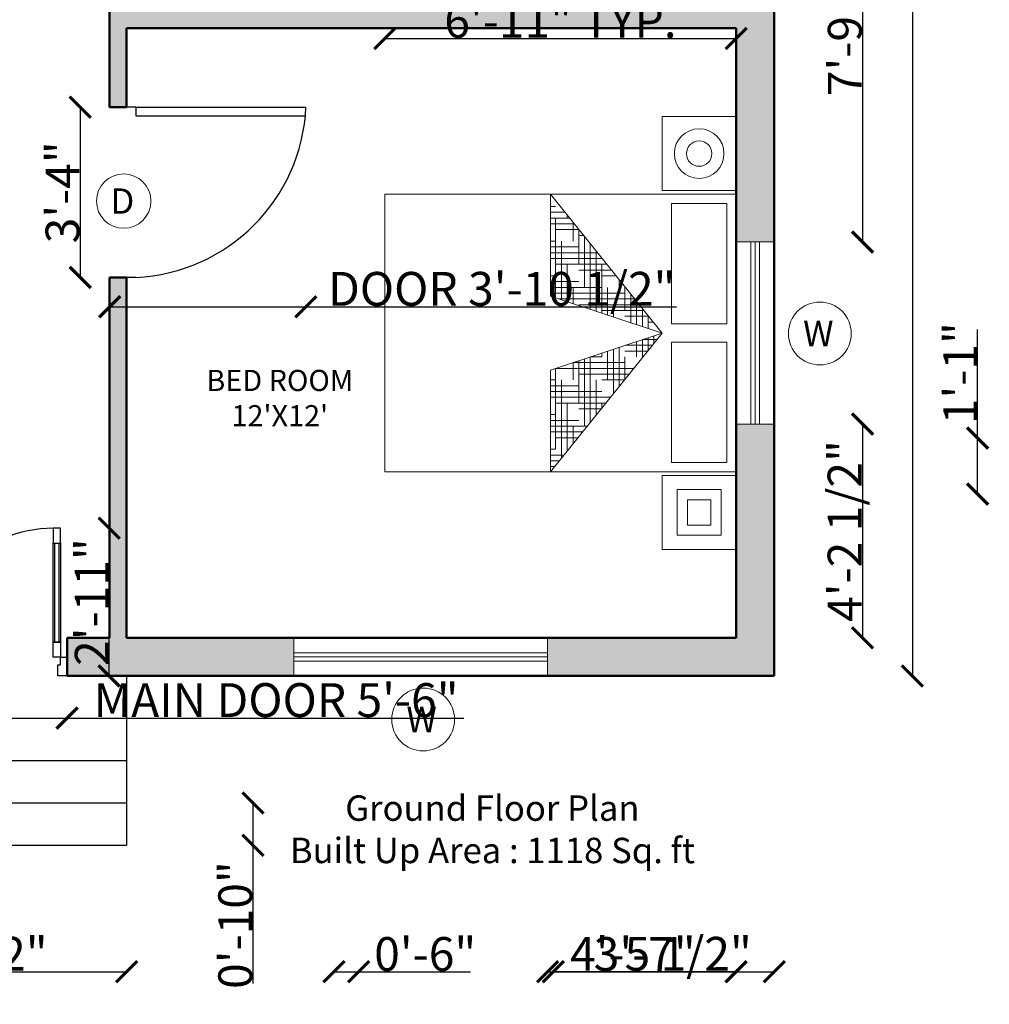
# Model space of a CAD drawing. Units: inches. Extents: x 2169 to 2662, y 1518 to 2151.
# Tile 3 of 6: x 2398 to 2627, y 1518 to 1751. Entities that reach past the tile are written whole.
import ezdxf

# ---------------------------------------------------------------- set-up
doc = ezdxf.new("R2010")
doc.units = ezdxf.units.IN
for name, color, linetype, lineweight in [('A-ANNO-DIMS', 2, 'Continuous', 18), ('A-ANNO-SYMB', 7, 'Continuous', 18), ('A-ANNO-TEXT', 7, 'Continuous', 18), ('A-AREA-IDEN', 7, 'Continuous', 18), ('A-FURN', 8, 'Continuous', 18), ('A-WALL-PATT', 30, 'Continuous', 13), ('Doors', 240, 'Continuous', 30), ('Main Door', 150, 'Continuous', 30), ('Steps', 50, 'Continuous', 25), ('Walls', 7, 'Continuous', 50), ('Windows', 160, 'Continuous', 18)]:
    doc.layers.add(name, color=color, linetype=linetype, lineweight=lineweight)
doc.layers.add('A-Glaz', color=92, linetype='Continuous')
doc.styles.get("Standard").update_dxf_attribs({"font": 'arial.ttf'})
doc.dimstyles.get("Standard").update_dxf_attribs({"dimtxt": 8, "dimasz": 5, "dimexe": 0.18, "dimexo": 0.0625, "dimgap": 0.09, "dimtad": 1, "dimdec": 1, "dimzin": 0, "dimdsep": 46, "dimlunit": 4, "dimtxsty": 'Standard', "dimblk": 'ARCHTICK', "dimcen": 0.09, "dimse1": 1, "dimse2": 1, "dimadec": 0, "dimazin": 0, "dimtfac": 1, "dimtdec": 1, "dimtofl": 0, "dimtmove": 0, "dimatfit": 3, "dimfxl": 1, "dimtolj": 1, "dimtzin": 0, "dimarcsym": 0})

# ---------------------------------------------------------------- blocks, each defined once
blk = doc.blocks.new('_ArchTick')
at = {"color": 0, "linetype": 'ByBlock', "const_width": 0.15}
blk.add_lwpolyline([(-0.5, -0.5), (0.5, 0.5)], dxfattribs=at)
blk = doc.blocks.new('*D3')
at = {"layer": 'A-ANNO-DIMS', "color": 0, "lineweight": -2, "transparency": 16777216}
blk.add_line((2608.61, 2111.6), (2608.61, 1595.6), dxfattribs=at)
at = {"layer": 'Defpoints', "color": 0, "transparency": 16777216}
for p in [(2575.74, 2111.6), (2575.98, 1595.6), (2608.61, 1595.6)]:
    blk.add_point(p, dxfattribs=at)
at = {"layer": 'A-ANNO-DIMS', "color": 0, "lineweight": -2, "transparency": 16777216, "xscale": 5, "yscale": 5, "zscale": 5}
for p, rotation in [((2608.61, 2111.6), 90), ((2608.61, 1595.6), 270)]:
    blk.add_blockref('_ArchTick', p, dxfattribs=dict(at, rotation=rotation))
at = {"layer": 'A-ANNO-DIMS', "color": 0, "transparency": 16777216, "insert": (2604.43, 1853.6), "char_height": 8, "attachment_point": 5, "rotation": 90}
blk.add_mtext("\\A1;43'", dxfattribs=at)
blk = doc.blocks.new('A$C13CE0A17')
at = {"layer": 'A-Glaz'}
for p, q in [((0.01, 0.61), (0.01, 0.08)), ((0.03, 0.08), (0.03, 0.61))]:
    blk.add_line(p, q, dxfattribs=at)
blk.add_lwpolyline([(1.4, 0.08), (1.4, 0.61), (1.42, 0.61), (1.42, 0.08)], close=True, dxfattribs=at)
at = {"layer": 'Main Door'}
for p, q in [((0, 0.61), (0, 0.69)), ((0, 0.69), (0.04, 0.69)), ((0.04, 0.69), (0.04, 0.61)), ((0, 0.61), (0, 0.08)), ((0.04, 0.61), (0, 0.61)), ((0.04, 0.61), (0, 0.61)), ((0.03, 0.61), (0.01, 0.61)), ((0.04, 0.08), (0.04, 0.61)), ((0, 0.08), (0, 0)), ((0.04, 0.08), (0, 0.08)), ((0, 0.08), (0.04, 0.08)), ((0.01, 0.08), (0.03, 0.08)), ((0.04, 0), (0.04, 0.08)), ((-0.035, 0), (-0.035, -0.1)), ((0, 0), (-0.035, 0)), ((0, 0), (0.04, 0)), ((0, -0.04), (0, 0)), ((0.015, -0.04), (0, -0.04)), ((0.015, -0.05), (0.015, -0.04)), ((0.015, -0.1), (0.015, -0.05)), ((-0.035, -0.1), (0.015, -0.1))]:
    blk.add_line(p, q, dxfattribs=at)
for points in [[(1.39, 0.69), (1.39, 0.61), (1.43, 0.61), (1.43, 0.69)], [(1.39, 0.08), (1.39, 0.61), (1.43, 0.61), (1.43, 0.08)], [(1.39, 0), (1.39, 0.08), (1.43, 0.08), (1.43, 0)], [(1.43, 0), (1.465, 0), (1.465, -0.1), (1.415, -0.1), (1.415, -0.05), (1.415, -0.04), (1.43, -0.04)]]:
    blk.add_lwpolyline(points, close=True, dxfattribs=at)
blk.add_arc((1.3872, 0.017), 0.673, 89.7657, 181.4438, dxfattribs=at)
blk.add_ellipse((0.0389, 0.0511), major_axis=(0.6669, -0.1217), ratio=0.940794, start_param=0.11153, end_param=1.73917, dxfattribs=at)
blk = doc.blocks.new('*X16')
at = {"color": 0}
for p, q in [((20.25, 14.8125), (20.2772, 14.8125)), ((20.1739, 14.75), (20.2772, 14.75)), ((20.1875, 14.75), (20.1875, 14.7669)), ((20.199, 14.7812), (20.2772, 14.7812)), ((20.25, 14.3194), (20.25, 14.75)), ((20.1487, 14.7188), (20.2772, 14.7188)), ((20.1562, 14.625), (20.1562, 14.7281)), ((20.0938, 14.375), (20.0938, 14.6504)), ((20.0984, 14.6562), (20.125, 14.6562)), ((20.1236, 14.6875), (20.25, 14.6875)), ((20.125, 14.5), (20.125, 14.6893)), ((20.0625, 14.2573), (20.0625, 14.6116)), ((20.125, 14.5938), (20.2772, 14.5938)), ((20.2188, 14.3091), (20.2188, 14.625)), ((20.25, 14.625), (20.2772, 14.625)), ((20.023, 14.5625), (20.2772, 14.5625)), ((20.0312, 14.2469), (20.0312, 14.5727)), ((19.9727, 14.5), (20.25, 14.5)), ((19.9979, 14.5312), (20.2772, 14.5312)), ((20, 14.2366), (20, 14.5)), ((20.1875, 14.2987), (20.1875, 14.5)), ((19.9225, 14.4375), (20, 14.4375)), ((19.9476, 14.4688), (20.125, 14.4688)), ((20.25, 14.4375), (20.2772, 14.4375)), ((19.875, 14.25), (19.875, 14.3785)), ((19.9062, 14.375), (19.9062, 14.4174)), ((19.9688, 14.2262), (19.9688, 14.375)), ((20, 14.375), (20.2772, 14.375)), ((20.125, 14.4062), (20.2772, 14.4062)), ((20.1562, 14.2884), (20.1562, 14.375)), ((19.8438, 14.1848), (19.8438, 14.3397)), ((19.875, 14.3438), (20.2772, 14.3438)), ((19.7967, 14.2812), (20.125, 14.2812)), ((19.8125, 14.1744), (19.8125, 14.3008)), ((19.8219, 14.3125), (20.2291, 14.3125)), ((19.7465, 14.2188), (19.875, 14.2188)), ((19.75, 14.1537), (19.75, 14.2231)), ((19.7716, 14.25), (20, 14.25)), ((19.7812, 14.1641), (19.7812, 14.262)), ((19.9375, 14.2159), (19.9375, 14.25)), ((19.7213, 14.1875), (19.75, 14.1875)), ((19.7188, 14.0726), (19.7188, 14.1136)), ((19.7018, 14.0938), (19.7786, 14.0938)), ((19.7269, 14.0625), (19.8728, 14.0625)), ((19.75, 14.0338), (19.75, 14.1032)), ((19.7812, 13.9949), (19.7812, 14.0929)), ((19.8125, 14), (19.8125, 14.0825)), ((19.752, 14.0312), (19.875, 14.0312)), ((19.9062, 13.8396), (19.9062, 14.0514)), ((19.9375, 13.8007), (19.9375, 14.0411)), ((19.9688, 13.875), (19.9688, 14.0307)), ((20, 14), (20, 14.0204)), ((19.875, 13.8784), (19.875, 14)), ((19.875, 13.9688), (20.1557, 13.9688)), ((20, 14), (20.0614, 14)), ((20.0625, 13.6454), (20.0625, 13.9996)), ((20.0938, 13.625), (20.0938, 13.9893)), ((20.125, 13.75), (20.125, 13.9789)), ((20.1562, 13.875), (20.1562, 13.9686)), ((19.8275, 13.9375), (20.25, 13.9375)), ((19.8526, 13.9062), (20.125, 13.9062)), ((20.25, 13.5), (20.25, 13.9375)), ((19.8777, 13.875), (20, 13.875)), ((20.0312, 13.6842), (20.0312, 13.875)), ((20.125, 13.8438), (20.2772, 13.8438)), ((20.2188, 13.4511), (20.2188, 13.875)), ((20.25, 13.875), (20.2772, 13.875)), ((20, 13.8125), (20.2772, 13.8125)), ((19.9532, 13.7812), (20.2772, 13.7812)), ((19.9783, 13.75), (20.25, 13.75)), ((20, 13.723), (20, 13.75)), ((20.1875, 13.49), (20.1875, 13.75)), ((20.0035, 13.7188), (20.125, 13.7188)), ((20.25, 13.6875), (20.2772, 13.6875)), ((20.125, 13.6562), (20.2772, 13.6562)), ((20.0789, 13.625), (20.2772, 13.625)), ((20.104, 13.5938), (20.2772, 13.5938)), ((20.1562, 13.5288), (20.1562, 13.625)), ((20.1292, 13.5625), (20.25, 13.5625)), ((20.25, 13.5), (20.2772, 13.5)), ((20.2046, 13.4688), (20.2772, 13.4688)), ((20.2297, 13.4375), (20.2772, 13.4375)), ((20.2549, 13.4062), (20.2772, 13.4062))]:
    blk.add_line(p, q, dxfattribs=at)
blk = doc.blocks.new('MAT-P13')
for p, q in [((-1.17, 0), (-1.17, -0.4)), ((-1.17, 0), (-0.77, 0)), ((-0.77, 0), (-0.77, -0.4)), ((-0.75, 0), (0.75, 0)), ((-0.75, 0), (-0.75, -1.9)), ((0.75, 0), (0.75, -1.9)), ((0.77, 0), (1.17, 0)), ((0.77, 0), (0.77, -0.4)), ((1.17, 0), (1.17, -0.4)), ((-0.7, -0.05), (-0.7, -0.35)), ((-0.7, -0.05), (-0.05, -0.05)), ((-0.05, -0.35), (-0.05, -0.05)), ((0.05, -0.05), (0.7, -0.05)), ((0.05, -0.35), (0.05, -0.05)), ((0.7, -0.05), (0.7, -0.35)), ((-0.7, -0.35), (-0.05, -0.35)), ((0.05, -0.35), (0.7, -0.35)), ((-1.17, -0.4), (-0.77, -0.4)), ((-0.75, -1.0034), (0, -0.4)), ((0, -0.4), (-0.75, -1.0034)), ((0, -0.4), (-0.2, -1.0034)), ((0, -0.4), (0.2, -1.0034)), ((0, -0.4), (0.75, -1.0034)), ((0.77, -0.4), (1.17, -0.4)), ((-0.75, -1.0034), (-0.2, -1.0034)), ((0.2, -1.0034), (0.75, -1.0034)), ((0.75, -1.9), (-0.75, -1.9))]:
    blk.add_line(p, q)
for points in [[(0.8468, -0.0814), (1.0932, -0.0814), (1.0932, -0.3186), (0.8468, -0.3186)], [(0.9015, -0.1361), (1.0385, -0.1361), (1.0385, -0.2639), (0.9015, -0.2639)]]:
    blk.add_lwpolyline(points, close=True)
for radius in [0.1342, 0.0686]:
    blk.add_circle((-0.97, -0.2), radius)
at = {"xscale": -1, "rotation": 90}
blk.add_blockref('*X16', (14.1285, 19.2738), dxfattribs=at)
blk = doc.blocks.new('AP0B05')
for p, q in [((35, 100), (35, 880)), ((75, 100), (75, 878.9)), ((35, 100), (35, -20)), ((815, 100), (815, -20))]:
    blk.add_line(p, q)
blk.add_lwpolyline([(35, 100), (75, 100)])
blk.add_arc((-2.4, 62.6), 818.3, 2.6212, 87.3788)
blk = doc.blocks.new('GLAZING-43IN')
for p, q in [((-21.5, 1), (21.5, 1)), ((-21.5, 0), (21.5, 0)), ((-21.5, -1), (21.5, -1))]:
    blk.add_line(p, q)
blk = doc.blocks.new('OPENING-TAG-W')
blk.add_circle((0, 0), 7.42)
blk.add_text('W', height=6).set_placement((-3.96, -3))
blk = doc.blocks.new('OPENING-TAG-D')
blk.add_circle((0, 0), 6.43)
blk.add_text('D', height=6).set_placement((-3.13, -3))
blk = doc.blocks.new('*D37')
at = {"layer": 'A-ANNO-DIMS', "color": 0, "lineweight": -2, "transparency": 16777216}
for p, q in [((2418.98, 1682.79), (2465.34, 1682.79)), ((2465.34, 1682.79), (2552.88, 1682.79))]:
    blk.add_line(p, q, dxfattribs=at)
at = {"layer": 'Defpoints', "color": 0, "transparency": 16777216}
for p in [(2418.98, 1689.75), (2465.34, 1689.75), (2465.34, 1682.79)]:
    blk.add_point(p, dxfattribs=at)
at = {"layer": 'A-ANNO-DIMS', "color": 0, "lineweight": -2, "transparency": 16777216, "xscale": 5, "yscale": 5, "zscale": 5, "rotation": 180}
blk.add_blockref('_ArchTick', (2418.98, 1682.79), dxfattribs=at)
at = {"layer": 'A-ANNO-DIMS', "color": 0, "lineweight": -2, "transparency": 16777216, "xscale": 5, "yscale": 5, "zscale": 5}
blk.add_blockref('_ArchTick', (2465.34, 1682.79), dxfattribs=at)
at = {"layer": 'A-ANNO-DIMS', "color": 0, "transparency": 16777216, "insert": (2511.61, 1687.03), "char_height": 8, "attachment_point": 5}
blk.add_mtext('\\A1;DOOR 3\'-10 1/2"', dxfattribs=at)
blk = doc.blocks.new('*D38')
at = {"layer": 'A-ANNO-DIMS', "color": 0, "lineweight": -2, "transparency": 16777216}
blk.add_line((2412.02, 1729.93), (2412.02, 1689.75), dxfattribs=at)
at = {"layer": 'Defpoints', "color": 0, "transparency": 16777216}
for p in [(2418.98, 1729.93), (2412.02, 1689.75), (2418.98, 1689.75)]:
    blk.add_point(p, dxfattribs=at)
at = {"layer": 'A-ANNO-DIMS', "color": 0, "lineweight": -2, "transparency": 16777216, "xscale": 5, "yscale": 5, "zscale": 5}
for p, rotation in [((2412.02, 1729.93), 90), ((2412.02, 1689.75), 270)]:
    blk.add_blockref('_ArchTick', p, dxfattribs=dict(at, rotation=rotation))
at = {"layer": 'A-ANNO-DIMS', "color": 0, "transparency": 16777216, "insert": (2407.84, 1709.84), "char_height": 8, "attachment_point": 5, "rotation": 90}
blk.add_mtext('\\A1;3\'-4"', dxfattribs=at)
blk = doc.blocks.new('*D41')
at = {"layer": 'A-ANNO-DIMS', "color": 0, "lineweight": -2, "transparency": 16777216}
for p, q in [((2342.72, 1585.67), (2408.92, 1585.67)), ((2408.92, 1585.67), (2502.68, 1585.67))]:
    blk.add_line(p, q, dxfattribs=at)
at = {"layer": 'Defpoints', "color": 0, "transparency": 16777216}
for p in [(2342.72, 1595.6), (2408.92, 1595.6), (2408.92, 1585.67)]:
    blk.add_point(p, dxfattribs=at)
at = {"layer": 'A-ANNO-DIMS', "color": 0, "lineweight": -2, "transparency": 16777216, "xscale": 5, "yscale": 5, "zscale": 5, "rotation": 180}
blk.add_blockref('_ArchTick', (2342.72, 1585.67), dxfattribs=at)
at = {"layer": 'A-ANNO-DIMS', "color": 0, "lineweight": -2, "transparency": 16777216, "xscale": 5, "yscale": 5, "zscale": 5}
blk.add_blockref('_ArchTick', (2408.92, 1585.67), dxfattribs=at)
at = {"layer": 'A-ANNO-DIMS', "color": 0, "transparency": 16777216, "insert": (2458.3, 1589.9), "char_height": 8, "attachment_point": 5}
blk.add_mtext('\\A1;MAIN DOOR 5\'-6"', dxfattribs=at)
blk = doc.blocks.new('*D42')
at = {"layer": 'A-ANNO-DIMS', "color": 0, "lineweight": -2, "transparency": 16777216}
blk.add_line((2418.86, 1595.6), (2418.86, 1630.51), dxfattribs=at)
at = {"layer": 'Defpoints', "color": 0, "transparency": 16777216}
for p in [(2408.92, 1630.51), (2418.86, 1630.51), (2408.92, 1595.6)]:
    blk.add_point(p, dxfattribs=at)
at = {"layer": 'A-ANNO-DIMS', "color": 0, "lineweight": -2, "transparency": 16777216, "xscale": 5, "yscale": 5, "zscale": 5}
for p, rotation in [((2418.86, 1630.51), 90), ((2418.86, 1595.6), 270)]:
    blk.add_blockref('_ArchTick', p, dxfattribs=dict(at, rotation=rotation))
at = {"layer": 'A-ANNO-DIMS', "color": 0, "transparency": 16777216, "insert": (2414.75, 1613.06), "char_height": 8, "attachment_point": 5, "rotation": 90}
blk.add_mtext('\\A1;2\'-11"', dxfattribs=at)
blk = doc.blocks.new('*D44')
at = {"layer": 'A-ANNO-DIMS', "color": 0, "lineweight": -2, "transparency": 16777216}
blk.add_line((2483.98, 1746.17), (2566.98, 1746.17), dxfattribs=at)
at = {"layer": 'Defpoints', "color": 0, "transparency": 16777216}
for p in [(2483.98, 1761.5), (2566.98, 1761.5), (2566.98, 1746.17)]:
    blk.add_point(p, dxfattribs=at)
at = {"layer": 'A-ANNO-DIMS', "color": 0, "lineweight": -2, "transparency": 16777216, "xscale": 5, "yscale": 5, "zscale": 5, "rotation": 180}
blk.add_blockref('_ArchTick', (2483.98, 1746.17), dxfattribs=at)
at = {"layer": 'A-ANNO-DIMS', "color": 0, "lineweight": -2, "transparency": 16777216, "xscale": 5, "yscale": 5, "zscale": 5}
blk.add_blockref('_ArchTick', (2566.98, 1746.17), dxfattribs=at)
at = {"layer": 'A-ANNO-DIMS', "color": 0, "transparency": 16777216, "insert": (2525.48, 1750.34), "char_height": 8, "attachment_point": 5}
blk.add_mtext('\\A1;6\'-11" TYP.', dxfattribs=at)
blk = doc.blocks.new('*D55')
at = {"layer": 'A-ANNO-DIMS', "color": 0, "lineweight": -2, "transparency": 16777216}
blk.add_line((2462.45, 2141.45), (2522.45, 2141.45), dxfattribs=at)
at = {"layer": 'Defpoints', "color": 0, "transparency": 16777216}
for p in [(2522.45, 2141.45), (2462.45, 1604.6), (2522.45, 1604.6)]:
    blk.add_point(p, dxfattribs=at)
at = {"layer": 'A-ANNO-DIMS', "color": 0, "lineweight": -2, "transparency": 16777216, "xscale": 5, "yscale": 5, "zscale": 5, "rotation": 180}
blk.add_blockref('_ArchTick', (2462.45, 2141.45), dxfattribs=at)
at = {"layer": 'A-ANNO-DIMS', "color": 0, "lineweight": -2, "transparency": 16777216, "xscale": 5, "yscale": 5, "zscale": 5}
blk.add_blockref('_ArchTick', (2522.45, 2141.45), dxfattribs=at)
at = {"layer": 'A-ANNO-DIMS', "color": 0, "transparency": 16777216, "insert": (2492.45, 2145.63), "char_height": 8, "attachment_point": 5}
blk.add_mtext('\\A1;5\'-0"', dxfattribs=at)
blk = doc.blocks.new('*D56')
at = {"layer": 'A-ANNO-DIMS', "color": 0, "lineweight": -2, "transparency": 16777216}
blk.add_line((2342.72, 1525.75), (2422.98, 1525.75), dxfattribs=at)
at = {"layer": 'Defpoints', "color": 0, "transparency": 16777216}
for p in [(2342.72, 1555.6), (2422.98, 1555.6), (2422.98, 1525.75)]:
    blk.add_point(p, dxfattribs=at)
at = {"layer": 'A-ANNO-DIMS', "color": 0, "lineweight": -2, "transparency": 16777216, "xscale": 5, "yscale": 5, "zscale": 5, "rotation": 180}
blk.add_blockref('_ArchTick', (2342.72, 1525.75), dxfattribs=at)
at = {"layer": 'A-ANNO-DIMS', "color": 0, "lineweight": -2, "transparency": 16777216, "xscale": 5, "yscale": 5, "zscale": 5}
blk.add_blockref('_ArchTick', (2422.98, 1525.75), dxfattribs=at)
at = {"layer": 'A-ANNO-DIMS', "color": 0, "transparency": 16777216, "insert": (2382.85, 1529.98), "char_height": 8, "attachment_point": 5}
blk.add_mtext('\\A1;6\'-8 1/2"', dxfattribs=at)
blk = doc.blocks.new('*D61')
at = {"layer": 'A-ANNO-DIMS', "color": 0, "lineweight": -2, "transparency": 16777216}
blk.add_line((2596.83, 1655.1), (2596.83, 1604.6), dxfattribs=at)
at = {"layer": 'Defpoints', "color": 0, "transparency": 16777216}
for p in [(2566.98, 1655.1), (2566.98, 1604.6), (2596.83, 1604.6)]:
    blk.add_point(p, dxfattribs=at)
at = {"layer": 'A-ANNO-DIMS', "color": 0, "lineweight": -2, "transparency": 16777216, "xscale": 5, "yscale": 5, "zscale": 5}
for p, rotation in [((2596.83, 1655.1), 90), ((2596.83, 1604.6), 270)]:
    blk.add_blockref('_ArchTick', p, dxfattribs=dict(at, rotation=rotation))
at = {"layer": 'A-ANNO-DIMS', "color": 0, "transparency": 16777216, "insert": (2592.6, 1629.85), "char_height": 8, "attachment_point": 5, "rotation": 90}
blk.add_mtext('\\A1;4\'-2 1/2"', dxfattribs=at)
blk = doc.blocks.new('*D62')
at = {"layer": 'A-ANNO-DIMS', "color": 0, "lineweight": -2, "transparency": 16777216}
blk.add_line((2596.83, 1791.1), (2596.83, 1698.1), dxfattribs=at)
at = {"layer": 'Defpoints', "color": 0, "transparency": 16777216}
for p in [(2566.98, 1791.1), (2566.98, 1698.1), (2596.83, 1698.1)]:
    blk.add_point(p, dxfattribs=at)
at = {"layer": 'A-ANNO-DIMS', "color": 0, "lineweight": -2, "transparency": 16777216, "xscale": 5, "yscale": 5, "zscale": 5}
for p, rotation in [((2596.83, 1791.1), 90), ((2596.83, 1698.1), 270)]:
    blk.add_blockref('_ArchTick', p, dxfattribs=dict(at, rotation=rotation))
at = {"layer": 'A-ANNO-DIMS', "color": 0, "transparency": 16777216, "insert": (2592.65, 1744.6), "char_height": 8, "attachment_point": 5, "rotation": 90}
blk.add_mtext('\\A1;7\'-9"', dxfattribs=at)
blk = doc.blocks.new('*D64')
at = {"layer": 'A-ANNO-DIMS', "color": 0, "lineweight": -2, "transparency": 16777216}
blk.add_line((2522.45, 1525.75), (2575.98, 1525.75), dxfattribs=at)
at = {"layer": 'Defpoints', "color": 0, "transparency": 16777216}
for p in [(2522.45, 1595.6), (2575.98, 1595.6), (2575.98, 1525.75)]:
    blk.add_point(p, dxfattribs=at)
at = {"layer": 'A-ANNO-DIMS', "color": 0, "lineweight": -2, "transparency": 16777216, "xscale": 5, "yscale": 5, "zscale": 5, "rotation": 180}
blk.add_blockref('_ArchTick', (2522.45, 1525.75), dxfattribs=at)
at = {"layer": 'A-ANNO-DIMS', "color": 0, "lineweight": -2, "transparency": 16777216, "xscale": 5, "yscale": 5, "zscale": 5}
blk.add_blockref('_ArchTick', (2575.98, 1525.75), dxfattribs=at)
at = {"layer": 'A-ANNO-DIMS', "color": 0, "transparency": 16777216, "insert": (2549.21, 1529.98), "char_height": 8, "attachment_point": 5}
blk.add_mtext('\\A1;4\'-5 1/2"', dxfattribs=at)
blk = doc.blocks.new('*D77')
at = {"layer": 'A-ANNO-DIMS', "color": 0, "lineweight": -2, "transparency": 16777216}
blk.add_line((2566.98, 1525.75), (2523.78, 1525.75), dxfattribs=at)
at = {"layer": 'Defpoints', "color": 0, "transparency": 16777216}
for p in [(2523.78, 1876.6), (2566.98, 1876.6), (2523.78, 1525.75)]:
    blk.add_point(p, dxfattribs=at)
at = {"layer": 'A-ANNO-DIMS', "color": 0, "lineweight": -2, "transparency": 16777216, "xscale": 5, "yscale": 5, "zscale": 5, "rotation": 180}
blk.add_blockref('_ArchTick', (2523.78, 1525.75), dxfattribs=at)
at = {"layer": 'A-ANNO-DIMS', "color": 0, "lineweight": -2, "transparency": 16777216, "xscale": 5, "yscale": 5, "zscale": 5}
blk.add_blockref('_ArchTick', (2566.98, 1525.75), dxfattribs=at)
at = {"layer": 'A-ANNO-DIMS', "color": 0, "transparency": 16777216, "insert": (2545.38, 1529.93), "char_height": 8, "attachment_point": 5}
blk.add_mtext('\\A1;3\'-7"', dxfattribs=at)
blk = doc.blocks.new('*D78')
at = {"layer": 'A-ANNO-DIMS', "color": 0, "lineweight": -2, "transparency": 16777216}
for p, q in [((2393.13, 1748.6), (2393.13, 1792.94)), ((2393.13, 1729.93), (2393.13, 1748.6))]:
    blk.add_line(p, q, dxfattribs=at)
at = {"layer": 'Defpoints', "color": 0, "transparency": 16777216}
for p in [(2393.13, 1748.6), (2422.98, 1748.6), (2422.98, 1729.93)]:
    blk.add_point(p, dxfattribs=at)
at = {"layer": 'A-ANNO-DIMS', "color": 0, "lineweight": -2, "transparency": 16777216, "xscale": 5, "yscale": 5, "zscale": 5}
for p, rotation in [((2393.13, 1748.6), 90), ((2393.13, 1729.93), 270)]:
    blk.add_blockref('_ArchTick', p, dxfattribs=dict(at, rotation=rotation))
at = {"layer": 'A-ANNO-DIMS', "color": 0, "transparency": 16777216, "insert": (2388.9, 1773.27), "char_height": 8, "attachment_point": 5, "rotation": 90}
blk.add_mtext('\\A1;1\'-6 1/2"', dxfattribs=at)
blk = doc.blocks.new('*D81')
at = {"layer": 'A-ANNO-DIMS', "color": 0, "lineweight": -2, "transparency": 16777216}
for p, q in [((2624.02, 1651.77), (2624.02, 1677.47)), ((2624.02, 1638.55), (2624.02, 1651.77))]:
    blk.add_line(p, q, dxfattribs=at)
at = {"layer": 'Defpoints', "color": 0, "transparency": 16777216}
for p in [(2323.65, 1651.77), (2624.02, 1651.77), (2323.65, 1638.55)]:
    blk.add_point(p, dxfattribs=at)
at = {"layer": 'A-ANNO-DIMS', "color": 0, "lineweight": -2, "transparency": 16777216, "xscale": 5, "yscale": 5, "zscale": 5}
for p, rotation in [((2624.02, 1651.77), 90), ((2624.02, 1638.55), 270)]:
    blk.add_blockref('_ArchTick', p, dxfattribs=dict(at, rotation=rotation))
at = {"layer": 'A-ANNO-DIMS', "color": 0, "transparency": 16777216, "insert": (2619.91, 1667.12), "char_height": 8, "attachment_point": 5, "rotation": 90}
blk.add_mtext('\\A1;1\'-1"', dxfattribs=at)
blk = doc.blocks.new('*D86')
at = {"layer": 'A-ANNO-DIMS', "color": 0, "lineweight": -2, "transparency": 16777216}
for p, q in [((2471.98, 1525.75), (2477.81, 1525.75)), ((2477.81, 1525.75), (2504.25, 1525.75))]:
    blk.add_line(p, q, dxfattribs=at)
at = {"layer": 'Defpoints', "color": 0, "transparency": 16777216}
for p in [(2471.98, 1876.6), (2477.81, 1876.6), (2477.81, 1525.75)]:
    blk.add_point(p, dxfattribs=at)
at = {"layer": 'A-ANNO-DIMS', "color": 0, "lineweight": -2, "transparency": 16777216, "xscale": 5, "yscale": 5, "zscale": 5, "rotation": 180}
blk.add_blockref('_ArchTick', (2471.98, 1525.75), dxfattribs=at)
at = {"layer": 'A-ANNO-DIMS', "color": 0, "lineweight": -2, "transparency": 16777216, "xscale": 5, "yscale": 5, "zscale": 5}
blk.add_blockref('_ArchTick', (2477.81, 1525.75), dxfattribs=at)
at = {"layer": 'A-ANNO-DIMS', "color": 0, "transparency": 16777216, "insert": (2493.53, 1529.93), "char_height": 8, "attachment_point": 5}
blk.add_mtext('\\A1;0\'-6"', dxfattribs=at)
blk = doc.blocks.new('*D87')
at = {"layer": 'A-ANNO-DIMS', "color": 0, "lineweight": -2, "transparency": 16777216}
for p, q in [((2452.83, 1565.6), (2452.83, 1555.6)), ((2452.83, 1555.6), (2452.83, 1522.94))]:
    blk.add_line(p, q, dxfattribs=at)
at = {"layer": 'Defpoints', "color": 0, "transparency": 16777216}
for p in [(2422.98, 1565.6), (2422.98, 1555.6), (2452.83, 1555.6)]:
    blk.add_point(p, dxfattribs=at)
at = {"layer": 'A-ANNO-DIMS', "color": 0, "lineweight": -2, "transparency": 16777216, "xscale": 5, "yscale": 5, "zscale": 5}
for p, rotation in [((2452.83, 1565.6), 90), ((2452.83, 1555.6), 270)]:
    blk.add_blockref('_ArchTick', p, dxfattribs=dict(at, rotation=rotation))
at = {"layer": 'A-ANNO-DIMS', "color": 0, "transparency": 16777216, "insert": (2448.65, 1536.77), "char_height": 8, "attachment_point": 5, "rotation": 90}
blk.add_mtext('\\A1;0\'-10"', dxfattribs=at)

msp = doc.modelspace()

# ---------------------------------------------------------------- hatches: boundary and pattern name
at = {"layer": 'A-WALL-PATT', "transparency": 33554585}
h = msp.add_hatch(color=256, dxfattribs=at)
h.dxf.hatch_style = 1
h.paths.add_polyline_path([(2575.98, 2111.6), (2263.98, 2111.6), (2263.98, 2066.68), (2272.98, 2066.68), (2272.98, 2102.6), (2418.98, 2102.6), (2418.98, 1982.6), (2413.75, 1982.6), (2413.75, 1978.6), (2418.98, 1978.6), (2418.98, 1954.6), (2429.26, 1954.6), (2429.26, 1958.6), (2422.98, 1958.6), (2422.98, 2102.6), (2566.98, 2102.6), (2566.98, 2052.1), (2575.98, 2052.1)])
h.paths.add_polyline_path([(2575.98, 2009.1), (2566.98, 2009.1), (2566.98, 1997.84), (2566.98, 1958.6), (2467.98, 1958.6), (2467.98, 1950.67), (2471.98, 1950.67), (2471.98, 1954.6), (2566.98, 1954.6), (2566.98, 1947.83), (2575.98, 1947.83)])
h.paths.add_polyline_path([(2272.98, 2023.68), (2263.98, 2023.68), (2263.98, 1944.7), (2272.98, 1944.7), (2272.98, 1978.6), (2369.77, 1978.6), (2369.77, 1982.6), (2272.98, 1982.6)])
h.paths.add_polyline_path([(2272.98, 1882.6), (2370.48, 1882.6), (2370.48, 1886.6), (2272.98, 1886.6), (2272.98, 1921.26), (2263.98, 1921.26), (2263.98, 1841.55), (2272.98, 1841.55)])
h.paths.add_polyline_path([(2272.98, 1798.55), (2263.98, 1798.55), (2263.98, 1689.49), (2272.98, 1689.49)])
h.paths.add_polyline_path([(2272.98, 1646.49), (2263.98, 1646.49), (2263.98, 1595.6), (2281.85, 1595.6), (2281.85, 1604.6), (2272.98, 1604.6)])
h.paths.add_polyline_path([(2342.72, 1600.02), (2342.72, 1604.6), (2324.85, 1604.6), (2324.85, 1595.6), (2342.72, 1595.6)])
h.paths.add_polyline_path([(2462.45, 1604.6), (2408.92, 1604.6), (2408.92, 1595.6), (2462.45, 1595.6)])
h.paths.add_polyline_path([(2422.98, 1689.75), (2418.98, 1689.75), (2418.98, 1604.6), (2422.98, 1604.6)])
h.paths.add_polyline_path([(2575.98, 1655.1), (2566.98, 1655.1), (2566.98, 1643.84), (2566.98, 1604.6), (2522.45, 1604.6), (2522.45, 1595.6), (2575.98, 1595.6)])
h.paths.add_polyline_path([(2575.98, 1791.1), (2566.98, 1791.1), (2566.98, 1752.6), (2422.98, 1752.6), (2422.98, 1816.31), (2418.98, 1816.31), (2418.98, 1729.93), (2422.98, 1729.93), (2422.98, 1748.6), (2566.98, 1748.6), (2566.98, 1698.1), (2575.98, 1698.1)])
h.paths.add_polyline_path([(2575.98, 1883.38), (2566.98, 1883.38), (2566.98, 1876.6), (2506.75, 1876.6), (2506.75, 1872.6), (2566.98, 1872.6), (2566.98, 1834.1), (2575.98, 1834.1)])
h.paths.add_polyline_path([(2477.81, 1876.6), (2471.98, 1876.6), (2471.98, 1913.6), (2566.98, 1913.6), (2566.98, 1906.83), (2575.98, 1906.83), (2575.98, 1924.38), (2566.98, 1924.38), (2566.98, 1917.6), (2471.98, 1917.6), (2471.98, 1921.14), (2467.98, 1921.14), (2467.98, 1876.6), (2418.98, 1876.6), (2418.98, 1855.49), (2422.98, 1855.49), (2422.98, 1872.6), (2477.81, 1872.6)])

# ---------------------------------------------------------------- linework, layer by layer
at = {"layer": 'Steps'}
for p, q in [((2422.98, 1595.6), (2422.98, 1555.6)), ((2342.72, 1575.6), (2422.98, 1575.6)), ((2342.72, 1565.6), (2422.98, 1565.6)), ((2342.72, 1555.6), (2422.98, 1555.6))]:
    msp.add_line(p, q, dxfattribs=at)
at = {"layer": 'Walls'}
for p, q in [((2575.98, 2111.6), (2575.98, 1595.6)), ((2418.98, 1816.31), (2418.98, 1729.93)), ((2422.98, 1748.6), (2566.98, 1748.6)), ((2422.98, 1748.6), (2422.98, 1729.93)), ((2566.98, 1748.6), (2566.98, 1604.6)), ((2418.98, 1729.93), (2422.98, 1729.93)), ((2418.98, 1689.75), (2422.98, 1689.75)), ((2418.98, 1689.75), (2418.98, 1604.6)), ((2422.98, 1689.75), (2422.98, 1604.6)), ((2408.92, 1604.6), (2408.92, 1595.6)), ((2408.92, 1604.6), (2418.98, 1604.6)), ((2422.98, 1604.6), (2566.98, 1604.6)), ((2408.92, 1595.6), (2575.98, 1595.6))]:
    msp.add_line(p, q, dxfattribs=at)
at = {"layer": 'Windows'}
for p, q in [((2462.45, 1601.1), (2522.45, 1601.1)), ((2462.45, 1600.1), (2522.45, 1600.1)), ((2462.45, 1599.1), (2522.45, 1599.1))]:
    msp.add_line(p, q, dxfattribs=at)
for points in [[(2566.98, 1655.1), (2566.98, 1698.1), (2575.98, 1698.1), (2575.98, 1655.1)], [(2462.45, 1604.6), (2522.45, 1604.6), (2522.45, 1595.6), (2462.45, 1595.6)]]:
    msp.add_lwpolyline(points, close=True, dxfattribs=at)

# ---------------------------------------------------------------- block references
at = {"layer": 'A-ANNO-SYMB'}
for name, p in [('OPENING-TAG-D', (2422.3, 1707.76)), ('OPENING-TAG-W', (2586.75, 1676.48)), ('OPENING-TAG-W', (2493.05, 1585.32))]:
    msp.add_blockref(name, p, dxfattribs=at)
at = {"layer": 'A-FURN', "xscale": 43.68114050857687, "yscale": 43.68114050857687, "zscale": 43.68114050857687, "rotation": 270}
msp.add_blockref('MAT-P13', (2566.98, 1676.6), dxfattribs=at)
at = {"layer": 'Doors', "xscale": 0.0515184714856466, "yscale": 0.0515184714856466, "zscale": 0.0515184714856466, "rotation": 269.9999999999979}
msp.add_blockref('AP0B05', (2420.01, 1731.74), dxfattribs=at)
at = {"layer": 'Main Door', "xscale": 44.13700514456166, "yscale": 44.13700514456166, "zscale": 44.13700514456166}
msp.add_blockref('A$C13CE0A17', (2344.26, 1600.02), dxfattribs=at)
at = {"layer": 'Windows', "rotation": 89.99999999999991}
msp.add_blockref('GLAZING-43IN', (2571.48, 1676.6), dxfattribs=at)

# ---------------------------------------------------------------- texts
at = {"layer": 'A-ANNO-TEXT', "insert": (2449.66, 1567.39), "char_height": 6, "attachment_point": 1}
msp.add_mtext_dynamic_manual_height_columns('\\pxqc;Ground Floor Plan\\PBuilt Up Area : 1118 Sq. ft', width=119.4686, gutter_width=12.5, heights=[18.75], dxfattribs=at)
at = {"layer": 'A-AREA-IDEN', "insert": (2427.58, 1667.9), "char_height": 5, "attachment_point": 1}
msp.add_mtext_dynamic_manual_height_columns("\\pxqc;BED ROOM\\P12'X12'", width=63.1797, gutter_width=12.5, heights=[0], dxfattribs=at)

# ---------------------------------------------------------------- dimensions: what is measured, and where the dimension line sits
at = {"layer": 'A-ANNO-DIMS'}
for base, p1, p2, picture, middle in [((2522.45, 2141.45), (2462.45, 1604.6), (2522.45, 1604.6), '*D55', (2492.45, 2145.63)), ((2477.81, 1525.75), (2471.98, 1876.6), (2477.81, 1876.6), '*D86', (2493.53, 1529.93)), ((2523.78, 1525.75), (2566.98, 1876.6), (2523.78, 1876.6), '*D77', (2545.38, 1529.93)), ((2575.98, 1525.75), (2522.45, 1595.6), (2575.98, 1595.6), '*D64', (2549.21, 1529.98)), ((2422.98, 1525.75), (2342.72, 1555.6), (2422.98, 1555.6), '*D56', (2382.85, 1529.98))]:
    dim = msp.add_linear_dim(base=base, p1=p1, p2=p2, dimstyle='Standard', override={"dimdec": 1, "dimlfac": 1, "dimrnd": 0, "dimzin": 1, "dimdsep": 46, "dimlunit": 4, "dimfrac": 2}, dxfattribs=at)
    dim.commit()
    dim.dimension.update_dxf_attribs({"geometry": picture, "text_midpoint": middle})
for base, p1, p2, angle, override, picture, middle in [((2608.61, 1595.6), (2575.74, 2111.6), (2575.98, 1595.6), 90, {"dimclrd": 0, "dimclre": 0, "dimclrt": 0}, '*D3', (2604.43, 1853.6)), ((2393.13, 1748.6), (2422.98, 1729.93), (2422.98, 1748.6), 90, {"dimdec": 1, "dimlfac": 1, "dimrnd": 0, "dimzin": 1, "dimdsep": 46, "dimlunit": 4, "dimfrac": 2}, '*D78', (2388.9, 1773.27)), ((2596.83, 1698.1), (2566.98, 1791.1), (2566.98, 1698.1), 270, {"dimdec": 1, "dimlfac": 1, "dimrnd": 0, "dimzin": 1, "dimdsep": 46, "dimlunit": 4, "dimfrac": 2}, '*D62', (2592.65, 1744.6)), ((2412.02, 1689.75), (2418.98, 1729.93), (2418.98, 1689.75), 270, {"dimdec": 1, "dimlfac": 1, "dimrnd": 0, "dimzin": 1, "dimdsep": 46, "dimlunit": 4, "dimfrac": 2}, '*D38', (2407.84, 1709.84)), ((2624.02, 1651.77), (2323.65, 1638.55), (2323.65, 1651.77), 90, {"dimdec": 1, "dimlfac": 1, "dimrnd": 0, "dimzin": 1, "dimdsep": 46, "dimlunit": 4, "dimfrac": 2}, '*D81', (2619.91, 1667.12)), ((2596.83, 1604.6), (2566.98, 1655.1), (2566.98, 1604.6), 270, {"dimdec": 1, "dimlfac": 1, "dimrnd": 0, "dimzin": 1, "dimdsep": 46, "dimlunit": 4, "dimfrac": 2}, '*D61', (2592.6, 1629.85)), ((2418.86, 1630.51), (2408.92, 1595.6), (2408.92, 1630.51), 90, {"dimdec": 1, "dimlfac": 1, "dimrnd": 0, "dimzin": 1, "dimdsep": 46, "dimlunit": 4, "dimfrac": 2}, '*D42', (2414.75, 1613.06)), ((2452.83, 1555.6), (2422.98, 1565.6), (2422.98, 1555.6), 270, {"dimdec": 1, "dimlfac": 1, "dimrnd": 0, "dimzin": 1, "dimdsep": 46, "dimlunit": 4, "dimfrac": 2}, '*D87', (2448.65, 1536.77))]:
    dim = msp.add_linear_dim(base=base, p1=p1, p2=p2, angle=angle, dimstyle='Standard', override=override, dxfattribs=at)
    dim.commit()
    dim.dimension.update_dxf_attribs({"geometry": picture, "text_midpoint": middle})
for base, p1, p2, text, picture, middle in [((2566.98, 1746.17), (2483.98, 1761.5), (2566.98, 1761.5), '<> TYP.', '*D44', (2525.48, 1750.34)), ((2465.34, 1682.79), (2418.98, 1689.75), (2465.34, 1689.75), 'DOOR <>', '*D37', (2511.61, 1687.03)), ((2408.92, 1585.67), (2342.72, 1595.6), (2408.92, 1595.6), 'MAIN DOOR <>', '*D41', (2458.3, 1589.9))]:
    dim = msp.add_linear_dim(base=base, p1=p1, p2=p2, text=text, dimstyle='Standard', override={"dimdec": 1, "dimlfac": 1, "dimrnd": 0, "dimzin": 1, "dimdsep": 46, "dimlunit": 4, "dimfrac": 2}, dxfattribs=at)
    dim.commit()
    dim.dimension.update_dxf_attribs({"geometry": picture, "text_midpoint": middle})

doc.saveas('drawing.dxf')
